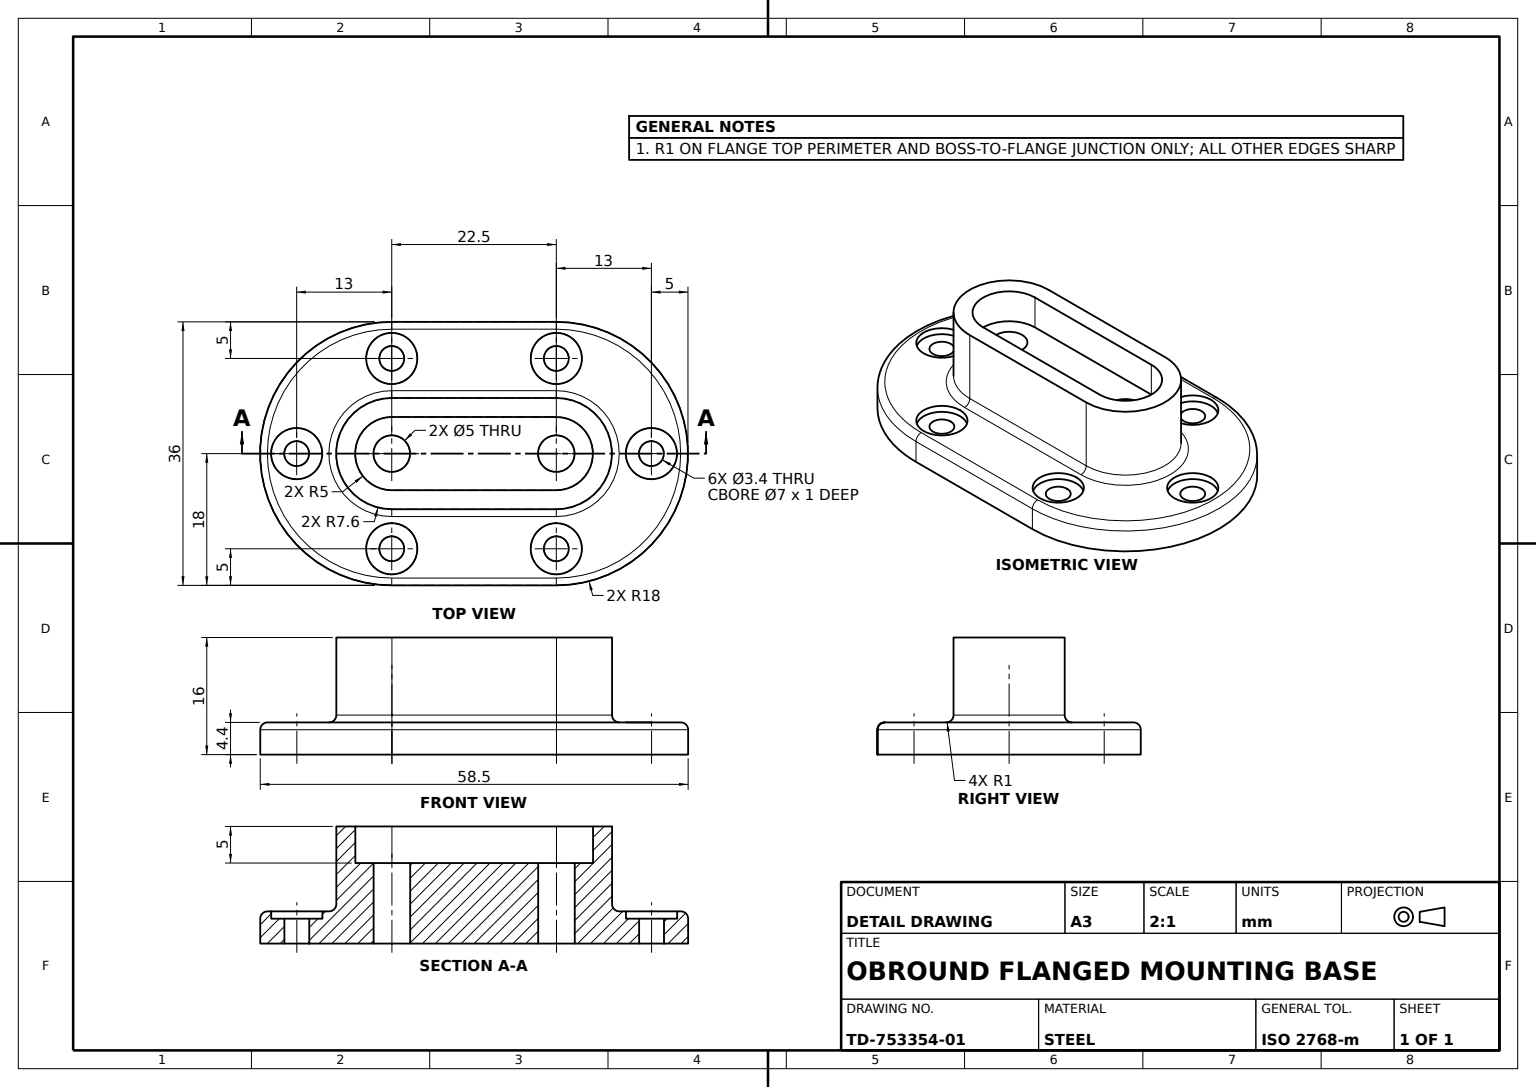
SolidWorks part; units mm, degrees
material "Plain Carbon Steel"
ref_plane "Front Plane" through (0, 0, 0) normal (0, 0, 1) x (1, 0, 0)
ref_plane "Top Plane" through (0, 0, 0) normal (0, 1, 0) x (1, 0, 0)
ref_plane "Right Plane" through (0, 0, 0) normal (1, 0, 0) x (0, 0, -1)
sketch "Base Flange Sketch" plane through (0, 0, 0) normal (0, 1, 0) x (1, 0, 0)
  line L0 (11.25, 0) -> (-11.25, 0) construction
  line L1 (11.25, -18) -> (-11.25, -18)
  line L2 (11.25, 18) -> (-11.25, 18)
  line L3 (-184.6865, 0) -> (9049.6365, 0) construction
  line L4 (0, -184.6865) -> (0, 9049.6365) construction
  arc A0 (11.25, -18) -> (11.25, 18) centre (11.25, 0) ccw
  arc A1 (-11.25, 18) -> (-11.25, -18) centre (-11.25, 0) ccw
  point P3 (0, 0)
  dimension "D2" = 18
  dimension "D1" = 22.5
extrude "Oval Base Flange" add sketch "Base Flange Sketch" along normal blind 4.4
sketch "Oval Boss Sketch" plane through (0, 4.4, 0) normal (0, 1, 0) x (1, 0, 0)
  line L0 (-11.25, 0) -> (11.25, 0) construction
  line L1 (-11.25, 7.6) -> (11.25, 7.6)
  line L2 (-11.25, -7.6) -> (11.25, -7.6)
  arc A0 (-11.25, 7.6) -> (-11.25, -7.6) centre (-11.25, 0) ccw
  arc A1 (11.25, -7.6) -> (11.25, 7.6) centre (11.25, 0) ccw
  point P3 (0, 0)
  dimension "D2" = 7.6
  dimension "D1" = 22.5
extrude "Raised Oval Boss" add sketch "Oval Boss Sketch" along normal blind 11.6
sketch "Oval Pocket Sketch" plane through (0, 16, 0) normal (0, 1, 0) x (1, 0, 0)
  line L0 (-11.25, 0) -> (11.25, 0) construction
  line L1 (-11.25, 5) -> (11.25, 5)
  line L2 (-11.25, -5) -> (11.25, -5)
  arc A0 (-11.25, 5) -> (-11.25, -5) centre (-11.25, 0) ccw
  arc A1 (11.25, -5) -> (11.25, 5) centre (11.25, 0) ccw
  point P3 (0, 0)
  dimension "D2" = 5
  dimension "D1" = 22.5
extrude "Oval Pocket R5" cut sketch "Oval Pocket Sketch" against normal blind 5
sketch "Counterbore Sketch" plane through (0, 4.4, 0) normal (0, 1, 0) x (1, 0, 0)
  line L0 (-11.25, 0) -> (11.25, 0) construction
  line L1 (-11.25, 13) -> (11.25, 13) construction
  line L2 (-11.25, -13) -> (11.25, -13) construction
  line L3 (-1000, 0) -> (49000, 0) construction
  line L4 (-11.25, 19.958) -> (-11.25, -20.5769) construction
  line L5 (11.25, 20.7626) -> (11.25, -22.0003) construction
  line L6 (0, -8.8) -> (0, 8.8) construction
  line L7 (-8.8, 0) -> (8.8, 0) construction
  line L8 (0, 19.0049) -> (0, -19.7722) construction
  arc A0 (-11.25, 13) -> (-11.25, -13) centre (-11.25, 0) ccw construction
  arc A1 (11.25, -13) -> (11.25, 13) centre (11.25, 0) ccw construction
  circle A2 centre (-11.25, 13) radius 3.5
  circle A3 centre (11.25, 13) radius 3.5
  circle A4 centre (11.25, -13) radius 3.5
  circle A5 centre (-11.25, -13) radius 3.5
  circle A6 centre (-24.25, 0) radius 3.5
  circle A7 centre (24.25, 0) radius 3.5
  point P3 (0, 0)
  dimension "D2" = 13
  dimension "D3" = 7
  dimension "D4" = 7
  dimension "D1" = 22.5
extrude "Mounting Hole Counterbores" cut sketch "Counterbore Sketch" against normal blind 1
sketch "Mounting Holes Sketch" plane through (0, 3.4, 0) normal (0, 1, 0) x (1, 0, 0)
  line L0 (-1000, 0) -> (49000, 0) construction
  line L1 (0, -1000) -> (0, 49000) construction
  line L2 (-11.25, -987) -> (-11.25, 49013) construction
  line L3 (11.25, -987) -> (11.25, 49013) construction
  circle A0 centre (-11.25, 13) radius 1.7
  circle A1 centre (11.25, 13) radius 1.7
  circle A2 centre (11.25, -13) radius 1.7
  circle A3 centre (-11.25, -13) radius 1.7
  circle A4 centre (-24.25, 0) radius 1.7
  circle A5 centre (24.25, 0) radius 1.7
  dimension "D1" = 3.4
  dimension "D2" = 3.4
extrude "Mounting Holes Ø3.4" cut sketch "Mounting Holes Sketch" against normal blind 7
sketch "Through Slot Sketch" plane through (0, 11, 0) normal (0, 1, 0) x (1, 0, 0)
  circle A0 centre (-11.25, 0) radius 2.5
  circle A1 centre (11.25, 0) radius 2.5
  dimension "D1" = 5
extrude "Pocket Through Slot" cut sketch "Through Slot Sketch" against normal blind 15
fillet "Boss Root Fillet R1" radius 1 8 edges at (0, 4.4, -18) (29.25, 4.4, 0) (0, 4.4, 18) (-29.25, 4.4, 0) (0, 4.4, -7.6) (18.85, 4.4, 0) (0, 4.4, 7.6) (-18.85, 4.4, 0)
